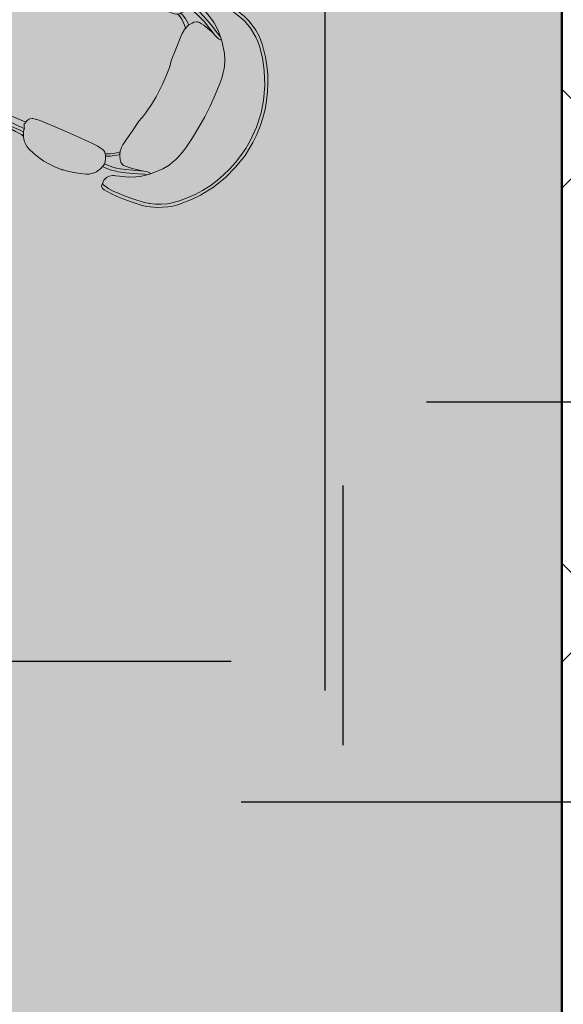
# Model space of a CAD drawing. Units: inches. Extents: x -466983 to 1020, y 324 to 318697.
# Tile 13 of 97: x 794 to 814, y 417 to 452. Entities that reach past the tile are written whole.
import ezdxf

# ---------------------------------------------------------------- set-up
doc = ezdxf.new("R2010")
doc.units = ezdxf.units.IN
doc.header["$MEASUREMENT"] = 0
for name, color, linetype, lineweight in [('A-ANNO-DIMS', 2, 'Continuous', 18), ('A-FLOR-PATT', 252, 'Continuous', 13), ('A-FURN', 8, 'Continuous', 18), ('A-WALL', 7, 'Continuous', 50)]:
    doc.layers.add(name, color=color, linetype=linetype, lineweight=lineweight)
doc.layers.add('K-Hatch', color=7, linetype='Continuous')
doc.styles.get("Standard").update_dxf_attribs({"font": 'arial.ttf'})
doc.dimstyles.get("Standard").update_dxf_attribs({"dimtxt": 6, "dimasz": 4, "dimexe": 3, "dimexo": 3, "dimgap": 0.09, "dimtad": 0, "dimtih": 1, "dimtoh": 1, "dimdec": 1, "dimzin": 0, "dimdsep": 46, "dimlunit": 3, "dimtxsty": 'Standard', "dimcen": 0.09, "dimadec": 0, "dimazin": 0, "dimtfac": 1, "dimtdec": 1, "dimtofl": 0, "dimtmove": 0, "dimatfit": 3, "dimfxl": 1, "dimtolj": 1, "dimtzin": 0, "dimarcsym": 0})

# ---------------------------------------------------------------- blocks, each defined once
blk = doc.blocks.new('CBV_11')
at = {"layer": 'K-Hatch'}
h = blk.add_hatch(color=256, dxfattribs=at)
h.dxf.hatch_style = 1
h.paths.add_polyline_path([(-178.4, 698.3), (-200.4, 717.9), (-207.1, 720), (-213, 721.7), (-231.8, 722.5), (-254.2, 721.5), (-275, 717.7), (-289.3, 712.5), (-316, 699.4), (-324.9, 694.8), (-295.8, 706.5), (-286.8, 709.3), (-277.1, 712.2), (-265.3, 715), (-258.1, 715.9), (-241.3, 718.1), (-228.8, 718), (-215.5, 715.7), (-208.8, 713.2), (-205.5, 711.6), (-203.9, 710.6), (-202.4, 709.7), (-195.4, 705.2), (-194.8, 704.5), (-190.4, 699.8), (-87.3, 570), (16.1, 440.3), (19.6, 435), (22.9, 426.4), (24.1, 422.9), (25.8, 412.3), (25.1, 398.9), (24.2, 394.5), (25.6, 399.8), (28.8, 418.8), (27.5, 432), (13.6, 457)])
h.paths.add_polyline_path([(-536, 213.1), (-639.3, 342.7), (-642.9, 348.1), (-646.2, 356.7), (-647.4, 360.2), (-649.1, 370.8), (-648.4, 384.2), (-645.7, 396.4), (-637.3, 419.1), (-631.8, 430), (-626.9, 438.8), (-622.1, 446.9), (-606.5, 469.3), (-631, 439.9), (-638.6, 427.4), (-646.5, 408.6), (-652.3, 388), (-655.6, 368.8), (-654.4, 355.7), (-649, 343.1), (-640.5, 330.7), (-448.6, 89.4), (-437.6, 77.7), (-424.8, 69.2), (-413.8, 65.9), (-392.4, 64.7), (-388.1, 65), (-394.5, 65), (-407.8, 67.4), (-417, 71.1), (-420.9, 73.4), (-427.9, 77.9), (-428.5, 78.6), (-432.9, 83.2)])
for p, q in [((259, 150.4), (259, 150.4)), ((345.2, 98.6), (344, 99.3)), ((349.3, 96), (349.2, 96.1)), ((478.6, -6.2), (478.7, -6.3)), ((644.9, -391.7), (644.8, -391.9)), ((-99, -470.6), (-98.6, -470.7)), ((4, -570.8), (3.9, -570.4)), ((96.9, -581.8), (98.6, -582.5)), ((157.6, -594.8), (157.4, -595)), ((239.9, -716.7), (240.2, -716.7))]:
    blk.add_line(p, q)
for points in [[(-16.4, 313.8), (-16.1, 314.2), (2.3, 340.9), (8.8, 352.7), (9, 353), (14.8, 365.2), (18.6, 375.8), (20.5, 381.1), (22.4, 386.6), (24.2, 394.5), (25.1, 398.9), (25.8, 412.3), (24.1, 422.9), (22.9, 426.4), (19.6, 435), (16.1, 440.3), (-87.3, 570), (-190.4, 699.8), (-194.8, 704.5), (-195.4, 705.2), (-202.4, 709.7), (-203.9, 710.6), (-208.8, 713.2), (-215.5, 715.7), (-228.8, 718), (-241.3, 718.1), (-258.1, 715.9), (-265.3, 715), (-277.1, 712.2), (-286.8, 709.3), (-295.8, 706.5), (-324.9, 694.8), (-347.4, 685.7), (-397.3, 660.4), (-444.8, 630.8), (-480.8, 604.2), (-497.4, 590.5), (-534.5, 556.2), (-554.4, 535.5), (-590.2, 492.6), (-603.5, 473.5), (-606.5, 469.3), (-622.1, 446.9), (-626.9, 438.8), (-631.8, 430), (-637.3, 419.1), (-645.7, 396.4), (-648.4, 384.2), (-649.1, 370.8), (-647.4, 360.2), (-646.2, 356.7), (-642.9, 348.1), (-639.3, 342.7), (-536, 213.1), (-432.9, 83.2), (-428.5, 78.6), (-427.9, 77.9), (-420.9, 73.4), (-417, 71.1), (-407.8, 67.4), (-394.5, 65), (-388.1, 65), (-382, 64.9), (-376.6, 65.6), (-368.3, 66.6), (-367.7, 66.7), (-359.3, 67.5), (-346.5, 70.4), (-345.9, 70.6), (-336.1, 73.3), (-327.3, 76.2), (-282.4, 94.4), (-275.6, 97.1), (-225.7, 122.4), (-178.3, 151.9), (-142.2, 178.6), (-125.6, 192.2), (-88.5, 226.6), (-68.7, 247.3), (-32.9, 290.2), (-16.4, 313.8), (-16.2, 314.2)], [(9, 353), (10.3, 354.9), (16.2, 365.1), (21.5, 376.3), (26.2, 388.3), (30.1, 400.3), (33.2, 412.3), (35.5, 424.1), (35.7, 431), (33.5, 442.1), (26.2, 456.4), (21.3, 463.1), (-173.2, 707.5), (-185, 718.7), (-200.1, 726), (-205.3, 726.9), (-216.4, 727.2), (-226.1, 726.9), (-241.2, 725.8), (-253.7, 723.9), (-264.9, 721.5), (-277.2, 717.9), (-288.3, 713.3), (-311.8, 701.8), (-324.9, 694.8), (-316, 699.4), (-289.3, 712.5), (-275, 717.7), (-254.2, 721.5), (-231.8, 722.5), (-213, 721.7), (-207.1, 720), (-200.4, 717.9), (-178.4, 698.3), (13.6, 457), (27.5, 432), (28.8, 418.8), (25.6, 399.8), (24.2, 394.5)], [(-203.9, 710.6), (-205.5, 711.6), (-208.8, 713.2)], [(-346.5, 70.4), (-349.3, 69.2), (-356.8, 67), (-372.9, 63.3), (-385.5, 61.5), (-398.1, 60.5), (-410.3, 60.2), (-421.5, 60.6), (-428.5, 61.9), (-441.8, 68.9), (-453.7, 80.2), (-456.3, 83.2), (-648.2, 324.6), (-653.1, 331.3), (-657.2, 338.3), (-662.3, 353.4), (-662.3, 363.4), (-659.9, 375.1), (-656.8, 387), (-652.8, 399), (-648.1, 410.9), (-642.7, 422.1), (-636.8, 432.3), (-630.4, 441.2), (-607, 469.6), (-603.5, 473.5)], [(-606.5, 469.3), (-631, 439.9), (-638.6, 427.4), (-646.5, 408.6), (-652.3, 388), (-655.6, 368.8), (-654.4, 355.7), (-649, 343.1), (-640.5, 330.7), (-448.6, 89.4), (-437.6, 77.7), (-424.8, 69.2), (-413.8, 65.9), (-392.4, 64.7), (-388.1, 65)], [(-50.1, 67.5), (-23.5, 87.9), (-9.9, 97.6), (3.8, 107.1), (17.8, 116.4), (31.9, 125.3), (60.6, 142.4), (89.9, 158.3), (119.5, 173.3), (135, 179.9), (142.8, 182.8), (151, 184.8), (159.6, 185.9), (175.9, 186.9), (181, 186.7)], [(46.8, 133.3), (53.6, 137.3), (58.1, 140), (60.8, 141.6), (71.5, 147.3), (71.5, 147.3), (75.4, 149.5), (86.9, 155.7), (90, 157.4), (100.5, 162.5), (100.5, 162.6), (112.3, 168.5), (118.5, 171.5), (121.5, 172.9), (121.5, 172.9), (121.6, 172.9), (124.8, 174.4), (126.7, 175.2), (131.7, 177.5), (133.5, 178.2), (133.6, 178.2), (139.5, 180.3), (143.1, 181.6), (144.9, 182), (148.5, 182.9), (151.1, 183.5), (151.4, 183.6), (155.5, 184.6), (157.4, 184.8), (163.9, 185.7), (168.2, 186.2), (170.2, 186.3), (175.4, 186.4), (175.6, 186.4), (175.8, 186.4), (179.6, 186.5), (181.7, 186.3), (187.4, 185.9), (192.1, 185.5), (192.4, 185.5), (192.9, 185.4), (196.6, 184.9), (199.1, 184.5), (203, 183.5), (203.6, 183.4), (204.9, 183.1), (206.1, 182.8), (206.2, 182.8), (206.9, 182.5), (210.6, 181.4), (212.8, 180.8), (213.1, 180.7), (213.6, 180.5), (215.8, 179.8), (217.2, 179.4), (219, 178.7), (225, 176.1), (225.2, 176), (225.4, 175.9), (228.9, 174.4), (230.6, 173.5), (239.3, 168.6), (259, 150.4), (261.9, 146.4), (265.2, 141.7), (271.3, 132.8), (271.8, 133.4)], [(268, 169.8), (264.7, 172.2), (256.3, 176.5), (245.7, 180.3), (233.5, 183.5), (219.5, 185.8), (204.9, 187.1), (190.5, 187.3), (181, 186.7), (184.6, 186.6), (192.1, 185.5)], [(215.8, 179.8), (224.2, 178.5), (244.5, 172), (258.1, 164.6), (259.6, 163.4)], [(325.2, 88.8), (320.7, 95.5), (312.8, 106.8), (299.7, 124.6), (287.2, 140.3), (277.4, 151.6), (268.4, 160.4), (262.4, 164.5), (259.6, 163.6), (268, 169.8), (268.8, 170.4), (273.2, 169.7), (281.2, 162.9), (287.4, 156.5), (292.6, 150.4), (299.8, 141.9), (315.6, 121.4), (329.6, 101.6), (335.5, 92.9)], [(259.6, 163.6), (259.6, 163.4), (260.3, 157.9), (264.5, 147.6), (271, 134.8), (273.6, 130.4), (280, 119.4), (306, 80.1)], [(58.1, 140), (55.3, 138.4), (46.8, 133.3), (43.3, 131.2), (32.8, 125), (30.4, 123.5), (28, 122), (23.4, 119.1), (14, 112.9), (5.4, 107.3), (1.3, 104.5), (-2.9, 101.6), (-9.4, 97), (-9.5, 96.9), (-21, 88.8), (-24.8, 86), (-28.5, 83.3), (-36.4, 77.2), (-38.8, 75.4), (-45.1, 70.6), (-49.7, 67), (-54.2, 63.4), (-56, 61.9), (-62.5, 56.6), (-75.5, 45.6), (-77.3, 44), (-77.4, 44)], [(346.5, 95.7), (344, 99.3), (342.7, 101.1), (342.4, 101.6), (329.1, 118.9), (319.4, 130.1), (312.4, 136.8), (292.6, 150.4)], [(457.4, -155.4), (455.9, -155.5), (454.8, -155.5), (454.6, -155.5), (454.5, -155.5), (450.3, -155.2), (448.8, -154.8), (444.9, -153.5), (441.6, -151.7), (437.3, -148.8), (429.3, -140.4), (425.9, -136.3), (421.6, -130.7), (411.3, -116.8), (398.5, -99.2), (386.7, -82.7), (374.5, -65.3), (362.5, -47.8), (339.1, -12.8), (318.2, 19.8), (307.7, 36.3), (302.4, 46.9), (301.4, 48.8), (298.5, 55.5), (297.9, 58.1), (297.8, 65.2), (298.5, 67.6), (301, 75.1), (306, 80.1), (307.5, 81.6), (308.1, 82), (307.8, 84), (308.9, 85.7), (310.4, 86.8), (312.8, 87.1), (320.3, 87.9), (323, 87.9), (324.8, 88.6), (325.2, 88.8), (330.7, 91.3), (335.5, 92.9), (337.7, 93.7), (344.7, 95.5), (346.5, 95.7), (349.3, 96), (349.8, 96), (359.2, 96.9), (368.2, 95.8), (377.2, 93.8), (385.7, 90.7), (393.6, 86.2), (410.4, 73.5), (416, 68.7), (426.3, 59.8), (441.3, 45.2), (454.8, 29), (467.2, 12.1), (478.3, -5.7), (478.6, -6.2), (478.6, -6.3), (479, -7), (481, -10.8), (488.2, -24.1), (496, -43.4), (503.1, -63.4), (508.5, -83.5), (509.8, -91.8), (509.7, -100.3), (508.6, -108.6), (506.6, -116.7), (503.3, -124.2), (500, -131.2), (494.1, -139.1), (490.8, -143.5), (486.4, -147), (485.6, -147.6), (485.6, -147.6)], [(349.8, 96), (347.9, 98), (342.9, 101.1), (342.7, 101.1)], [(-217.7, -216.8), (-218.7, -214.8), (-221.6, -206), (-223.5, -195.1), (-224.4, -170.3), (-223.2, -156.5), (-220.9, -142.4), (-219, -134.5), (-218.9, -134.4), (-218.9, -134.2), (-217.3, -125.9), (-215.2, -117.7), (-212.7, -109.9), (-212.1, -108.4), (-207.7, -98.2), (-203.6, -90.8), (-196.4, -80.6), (-191.3, -74), (-180.9, -61.1), (-170.2, -48.3), (-159.1, -35.9), (-159.1, -35.8), (-148, -23.5), (-124.9, 0.7), (-113, 12.4), (-100.8, 23.9), (-88.5, 35.1), (-75.9, 46.2), (-63.1, 57), (-50.1, 67.5)], [(-214.7, -118), (-214.6, -117.8), (-212.4, -111.4), (-210.9, -107.7), (-210.4, -106.5), (-210.1, -105.7), (-209.4, -104.2), (-209, -103.5), (-206, -97.3), (-205.1, -95.8), (-204.7, -95), (-203.9, -93.8), (-203.5, -93.2), (-202.6, -91.5), (-202, -90.5), (-200.3, -88.1), (-199.3, -86.6), (-198.2, -84.9), (-198, -84.7), (-197.9, -84.5), (-192.8, -77.9), (-190.9, -75.4), (-190.5, -74.9), (-189.8, -74), (-186.5, -69.8), (-173.8, -54.2), (-170.7, -50.6), (-169.2, -48.8), (-167, -46.3), (-160.8, -39.1), (-147.5, -24.2), (-147.4, -24.1), (-147.3, -24), (-146.9, -23.6), (-146.4, -23.1), (-134, -9.8), (-127, -2.7), (-124.7, -0.3), (-124.4, -0.1), (-124.2, 0.2), (-123.2, 1.2), (-120.2, 4.2), (-106.2, 17.9), (-102.9, 20.9), (-101.4, 22.4), (-98.9, 24.6), (-91.9, 31.1), (-77.7, 43.7), (-77.6, 43.8), (-77.4, 44)], [(479, -7), (479.3, -7.2), (478.7, -6.3), (478.6, -6.3)], [(481, -10.8), (480.9, -9.4), (480, -8.1), (479.3, -7.2), (479.9, -7.7), (480, -8.1), (480, -8.6)], [(-212.1, -108.4), (-213.8, -111.2), (-223, -134.4), (-228.6, -157.2), (-231.3, -180.4), (-231, -201.3), (-228.1, -217.6), (-225.8, -223.3), (-226.1, -223.6), (-227.6, -226.1), (-224.9, -232.9), (-218.3, -243.6), (-212.6, -251.5), (-209.6, -255.8), (-197.1, -271.4), (-182.6, -288.2), (-173.4, -298.4), (-166.3, -306.1)], [(-143.8, -278.1), (-149.7, -271.9), (-151.2, -270.2), (-153.6, -267.6), (-153.7, -267.6), (-158.2, -262.7), (-179.1, -240.4), (-181.9, -237.4), (-184, -235.2), (-185.8, -233.2), (-188.4, -230.4), (-188.8, -230), (-189.2, -229.5), (-191, -227.5), (-192.6, -225.7), (-192.9, -225.2), (-193.3, -224.8), (-194.6, -223.3), (-196.5, -221), (-197, -220.3), (-197.5, -219.7), (-198.5, -218.3), (-200, -216.4), (-200.2, -216.2), (-201.3, -214.6), (-201.4, -214.5), (-203.2, -212), (-203.8, -211.2), (-204.4, -210.2), (-205.3, -208.8), (-206.1, -207.6), (-206.2, -207.4), (-206.3, -207.3), (-206.4, -207), (-206.6, -206.8), (-207.1, -206), (-207.5, -205.3), (-207.5, -205.2), (-207.6, -205.1), (-207.6, -205), (-208.1, -204.2), (-208.2, -204), (-208.3, -203.8), (-208.4, -203.7), (-208.7, -203.2), (-209.4, -202), (-209.4, -201.9), (-209.6, -201.7), (-210.3, -200.2), (-211.3, -198.2), (-211.5, -197.7), (-212.6, -194.8), (-213.7, -191.8), (-214, -190.9), (-215.6, -185.2), (-217, -180.3), (-217, -180.3), (-217, -180.3), (-217.6, -177.7), (-218.5, -172.7), (-218.9, -170.6), (-219, -169.1), (-219.2, -168.2), (-219.2, -167.9), (-219.3, -167.8), (-219.3, -166.9), (-219.6, -165), (-219.8, -163.4), (-220.2, -156.1), (-220.2, -148.7), (-219.6, -142.8), (-219.6, -142.2), (-219.6, -142), (-219.6, -141.7), (-219.5, -141.2), (-218.5, -134), (-217.9, -130.8), (-217.7, -129.5), (-217.7, -129.3), (-217.5, -128.7), (-217.5, -128.6), (-217.4, -128.4), (-217, -126.3), (-215, -118.8), (-214.9, -118.6), (-214.9, -118.5), (-214.7, -118), (-214.9, -118.5)], [(2.4, -563.5), (-3.3, -568.8), (-5, -573.7), (-2.4, -580.9), (5.2, -592.9), (5.7, -593.8), (18.8, -610.1), (45.9, -638.4), (68.4, -659.3), (96.5, -683.5), (112.7, -694.7), (124, -701.1), (147.3, -712), (166.9, -718.5), (179.8, -721.6), (199.9, -724.8), (239.8, -727.2), (268.3, -726.6), (296.4, -724), (325.3, -719.4), (352.9, -713), (380.3, -704.7), (407.4, -694.3), (433.1, -682.4), (458.3, -668.7), (482.6, -653.1), (505.7, -636), (542.7, -602.8), (575.4, -565.6), (602.5, -526.6), (625.7, -483.1), (643.9, -436.4), (652.7, -404.6), (661, -358.1), (662.3, -341.6), (662.3, -324.4), (657.8, -289.7), (648.3, -258), (641.9, -243.3), (624.1, -210.4), (611.5, -188.5), (598.9, -168.7), (586.8, -151.4), (569.2, -131.1), (563.8, -126.7), (556, -124), (545.5, -130.4)], [(155.2, -596.2), (151.6, -595.8), (147.4, -595.1), (129.4, -592.1), (123.7, -590.8), (98.6, -582.5), (97.8, -582.2), (96.9, -581.8), (74.8, -570.5), (62.9, -563.8), (52.4, -557.5), (46.9, -554.5), (42.7, -553), (37.7, -551.6), (36.8, -551.4), (31.7, -550), (21.6, -550.8), (19.3, -551.6), (10.7, -555.3), (9.9, -555.9), (4.7, -561.9), (2.4, -563.5), (3.7, -570.3), (4, -570.8), (6.8, -576.4), (8.9, -579.3), (10.2, -583.1), (17.3, -590.8), (22.7, -598.1), (36.7, -613.8), (53.2, -630.5), (71.6, -647.7), (77.1, -652.5), (77.9, -653.2), (88.3, -662.3), (97.4, -670.5), (112.3, -681.7), (138.1, -696.5), (170, -708.5), (185.7, -712.2), (201.4, -714.5), (240.2, -716.9), (281.9, -715.3), (330.8, -707.8), (377.8, -694.8), (416.2, -679.4), (459.2, -656.3), (499.4, -628.1), (521, -609.6), (541.3, -589.7), (560.1, -568.5), (577.1, -546.4), (593, -522.5), (607, -498.1), (619.2, -472.7), (629.8, -445.9), (638.3, -419.5), (645, -392), (649.6, -365.8), (651.8, -341.4), (651.9, -325.2), (649.9, -305.2), (646.3, -287), (640.9, -268.7), (640.2, -267.3), (639, -264.2), (633.6, -250.9), (617.4, -220.5), (602.1, -193.8), (587.3, -171.3), (580.6, -161.1), (567.7, -144.8), (566, -143.1), (564.1, -141.2), (554.6, -132.1), (554, -131.9), (550.5, -130.5), (549.7, -130.2), (547.6, -129.3), (545.5, -130.4), (545.4, -130.9), (538.4, -135.5), (532.9, -143.1), (531.5, -145.1), (528.5, -154.8), (529, -166.6), (529.5, -170.7), (531.1, -176.4), (534.9, -188.3), (538.2, -199.2), (543, -215.6), (547.1, -240.2), (547.6, -254.2), (546.4, -277.3), (546.2, -281.9), (545.7, -285.4), (545.4, -287.9), (545.4, -287.9), (545.3, -288.8), (545.3, -289.2), (544.3, -296.8), (542.7, -303.6), (537, -331.4), (528.9, -353.7)], [(454.6, -155.5), (454.7, -155.7), (455.1, -157.8), (455.5, -160), (455.6, -160.6), (455.6, -160.7), (456.7, -166.6), (457.5, -171.5), (458.2, -182.7), (458.6, -192.3), (458.1, -202.7), (457.9, -204.1)], [(457.4, -155.4), (457.4, -155.4), (466.4, -154.5), (471.9, -153.3), (475.6, -151.4), (481.8, -150.7), (486.4, -147), (489.4, -151.4), (501.8, -172.4), (506.9, -183.2), (511.5, -194.8), (517.3, -212.7), (523.5, -234.6), (529.9, -258.9), (536.2, -278.2), (545.2, -290)], [(461.9, -154.9), (462.2, -156.4), (462.6, -158.7), (462.7, -159.1), (462.7, -159.3), (463.8, -165.3), (464.7, -170.7), (465.4, -182.4), (465.8, -192.3), (465.4, -201.6)], [(494.1, -139.1), (498.2, -145.2), (508.4, -161.7), (516.9, -179.1), (519.8, -186.7), (527.6, -210), (534, -233), (538.1, -249.1), (543.9, -270.8), (546.4, -277.4)], [(549.7, -130.2), (547, -129.8), (545.4, -130.9)], [(-225.8, -223.3), (-218.8, -216.5), (-217.7, -216.8), (-213.1, -218.1), (-195.7, -231.2), (-175.3, -250.4), (-147.2, -280.1)], [(-159.9, -297.1), (-165.4, -291.2), (-181.5, -273.1), (-197.1, -254.2), (-203.8, -245.5), (-213.9, -230.9), (-219, -220.9), (-218.8, -216.5)], [(-212.6, -251.5), (-211.9, -253), (-204.6, -272.1), (-201.7, -277.7), (-192.5, -291.1), (-180.6, -305.8), (-175.6, -311.7), (-173.4, -314.3), (-171.3, -316.5)], [(49.6, -472.3), (49.5, -472.3), (49.1, -466.8), (46.3, -459.7), (42.7, -453.8), (36.7, -445.8), (32.2, -440.3), (21, -427.2), (-6.6, -395.6), (-20.8, -379.7), (-35.2, -364.1), (-64.1, -333.5), (-77.2, -319.8), (-92.5, -304.3), (-108.7, -288.6), (-115.6, -282.9), (-121.5, -278.5), (-131.9, -275.3), (-141.2, -276.5), (-143.8, -278.1), (-147.2, -280.1), (-148.4, -280.8), (-149.5, -281.9), (-150.1, -282.4), (-156.3, -292.9), (-159.1, -296.2), (-158.4, -292.9), (-155.5, -285.3), (-153.9, -281.9), (-151.3, -281.2), (-149.5, -281.9)], [(545.7, -285.4), (544.3, -287.1), (544, -287.5), (543.6, -287.7), (543.5, -287.7)], [(59.4, -477), (56.9, -476.1), (53.2, -474.4), (49.6, -472.8), (49.7, -473.8), (48.7, -479.4), (48, -481.2), (44.9, -489.9), (42.9, -494.4), (41, -497.8), (38.6, -502.4), (37.3, -504.2), (36.9, -504.7), (34.8, -506.8), (33.8, -507.4), (29.1, -510.5), (24.1, -512.8), (22.1, -513.7), (15.1, -516.8), (-0.5, -520.1), (-9, -519.9), (-17.2, -519.3), (-25.5, -517.5), (-33.3, -514.4), (-51.7, -504.6), (-69.5, -493.5), (-86.6, -481.2), (-95.4, -473.4), (-97.6, -471.5), (-98, -471.2), (-98.6, -470.7), (-101.4, -468.2), (-101.5, -468.1), (-102.3, -467.4), (-117.4, -452.7), (-131.1, -436.8), (-143.6, -419.9), (-154.4, -402.1), (-164.5, -383.6), (-172.5, -364.3), (-175.2, -355.6), (-176.8, -346.5), (-176.8, -337.4), (-175.1, -328.4), (-173.5, -321.4), (-172.7, -319.6), (-171.3, -316.5), (-167.5, -308.1), (-166.3, -306.1), (-163.8, -301.8), (-160.2, -297.5), (-159.9, -297.1), (-159.1, -296.2)], [(-175.6, -311.7), (-175.4, -312.6), (-174, -317.8), (-172.7, -319.6)], [(528.6, -354.6), (528.9, -353.7), (522.8, -365.4), (515.7, -377.3), (508.1, -388.2), (503.2, -394.5), (496, -403.1), (483, -417.1), (469.3, -430.9), (454.9, -444.7), (425.1, -471.8), (395, -496.8), (363.8, -520.6), (330.7, -543.5), (314.1, -554.4), (297.5, -564.7), (281, -574.1), (263.9, -582.5), (251.4, -587.6), (244.7, -589.7), (224.5, -595.3), (204.1, -597.7), (165.9, -597.3), (155.2, -596.2), (157.4, -595), (157.2, -592.9), (152.6, -587.1)], [(-101.4, -468.2), (-100.6, -469.4), (-101.3, -468.7), (-101.5, -468.1)], [(-98, -471.2), (-98.4, -471.1), (-98.9, -470.8), (-99.9, -470.3), (-100.5, -469.5), (-100.6, -469.4)], [(-97.6, -471.5), (-98.3, -471.4), (-98.9, -470.8)], [(90.8, -500.6), (86.1, -499.5), (84, -498.9), (73.3, -495), (70.3, -493.8), (55.2, -486.1), (48, -481.2)], [(99.2, -488.5), (98.9, -488.4), (88.6, -486.6), (78.5, -484.1), (68.6, -480.9), (59.4, -477), (58.2, -476.5), (57.8, -476.3), (49.6, -472.3), (49.6, -472.3), (49.6, -472.4), (49.6, -472.4), (49.6, -472.5), (49.6, -472.8)], [(147.4, -595.1), (145, -593.4), (134.3, -587.3), (109, -574.1), (88.3, -563.1), (68.7, -551.4), (57.7, -543.9), (47.9, -536.1), (44.1, -532.6), (29.2, -518.3), (24.1, -512.8), (24.1, -512.8)], [(33.8, -507.4), (37.2, -511.1), (50.6, -524.3), (64.4, -535.5), (70.8, -539.8), (90.6, -552.1), (111.2, -563.3), (124.8, -570.5), (137.6, -577.4), (152.6, -587)]]:
    blk.add_lwpolyline(points)
blk.add_lwpolyline([(536.2, -278.2, 0.060196), (503, -207.6), (501.6, -205.9), (497.9, -203.4), (490.4, -200.5), (481.7, -199.9), (471.1, -200.5), (466.7, -201.3), (465.7, -201.5), (464.5, -201.7), (461.1, -203), (457.9, -204.1), (457.5, -204.3), (457.5, -204.3), (454.5, -205.4), (446.6, -210), (444.1, -211.8), (435.9, -217.8), (427.5, -225.4), (419.3, -234.2), (396.7, -256.7), (369.9, -282.9), (360.7, -294.8), (359, -297.1), (344.2, -313.2), (323.9, -333.2), (301.6, -353), (288.9, -363.5), (265.5, -381.1), (241.1, -397.6), (216.3, -412.6), (192.3, -424.2), (160.7, -444.5), (123.2, -467.5), (113.9, -474), (106.2, -480.6), (103.9, -482.6), (100.1, -487.3), (99.2, -488.5), (96.5, -492), (94.1, -495.1), (91.8, -498.2), (91.4, -499.3), (90.8, -500.6), (90.3, -501.9), (88.1, -510.2), (87, -512.3), (85.3, -518.2), (85.1, -527), (85.8, -529.8), (88.9, -536.1, 0.065332), (140.4, -579.1)], format="xyb")
blk = doc.blocks.new('Garden Sofa')
at = {"xscale": -0.0109740885734132, "yscale": 0.0109740885734132, "zscale": 0.0109740885734132, "rotation": 100.5267845499335}
blk.add_blockref('CBV_11', (2467.574, 814.959), dxfattribs=at)
blk = doc.blocks.new('*D93')
at = {"layer": 'A-ANNO-DIMS', "color": 0, "lineweight": -2, "transparency": 16777216}
for p, q in [((808.966, 500.777), (818.266, 500.777)), ((815.266, 496.777), (815.266, 472.969)), ((815.266, 442.777), (815.266, 466.584)), ((808.966, 438.777), (818.266, 438.777))]:
    blk.add_line(p, q, dxfattribs=at)
at = {"layer": 'A-ANNO-DIMS', "color": 0, "transparency": 16777216}
for points in [[(814.599, 496.777), (815.933, 496.777), (815.266, 500.777)], [(814.599, 442.777), (815.933, 442.777), (815.266, 438.777)]]:
    blk.add_solid(points, dxfattribs=at)
at = {"layer": 'Defpoints', "color": 0, "transparency": 16777216}
for p in [(805.966, 500.777), (815.266, 500.777), (805.966, 438.777)]:
    blk.add_point(p, dxfattribs=at)
at = {"layer": 'A-ANNO-DIMS', "color": 0, "transparency": 16777216, "insert": (815.266, 469.777), "char_height": 6, "attachment_point": 5}
blk.add_mtext('\\A1;GARDEN SEAT 62', dxfattribs=at)
blk = doc.blocks.new('*D94')
at = {"layer": 'A-ANNO-DIMS', "color": 0, "lineweight": -2, "transparency": 16777216}
for p, q in [((753.135, 435.777), (753.135, 426.477)), ((805.966, 435.777), (805.966, 426.477)), ((757.135, 429.477), (775.163, 429.477)), ((801.966, 429.477), (783.938, 429.477))]:
    blk.add_line(p, q, dxfattribs=at)
at = {"layer": 'A-ANNO-DIMS', "color": 0, "transparency": 16777216}
for points in [[(757.135, 430.143), (757.135, 428.81), (753.135, 429.477)], [(801.966, 430.143), (801.966, 428.81), (805.966, 429.477)]]:
    blk.add_solid(points, dxfattribs=at)
at = {"layer": 'Defpoints', "color": 0, "transparency": 16777216}
for p in [(753.135, 438.777), (805.966, 438.777), (805.966, 429.477)]:
    blk.add_point(p, dxfattribs=at)
at = {"layer": 'A-ANNO-DIMS', "color": 0, "transparency": 16777216, "insert": (779.551, 429.477), "char_height": 6, "attachment_point": 5}
blk.add_mtext('\\A1;53', dxfattribs=at)
blk = doc.blocks.new('*D97')
at = {"layer": 'A-ANNO-DIMS', "color": 0, "lineweight": -2, "transparency": 16777216}
for p, q in [((823.929, 568.441), (802.329, 568.441)), ((805.329, 564.441), (805.329, 499.545)), ((805.329, 428.441), (805.329, 493.337)), ((823.929, 424.441), (802.329, 424.441))]:
    blk.add_line(p, q, dxfattribs=at)
at = {"layer": 'A-ANNO-DIMS', "color": 0, "transparency": 16777216}
for points in [[(804.662, 564.441), (805.996, 564.441), (805.329, 568.441)], [(804.662, 428.441), (805.996, 428.441), (805.329, 424.441)]]:
    blk.add_solid(points, dxfattribs=at)
at = {"layer": 'Defpoints', "color": 0, "transparency": 16777216}
for p in [(826.929, 568.441), (805.329, 424.441), (826.929, 424.441)]:
    blk.add_point(p, dxfattribs=at)
at = {"layer": 'A-ANNO-DIMS', "color": 0, "transparency": 16777216, "insert": (805.329, 496.441), "char_height": 6, "attachment_point": 5}
blk.add_mtext('\\A1;BIKE 144', dxfattribs=at)

msp = doc.modelspace()

# ---------------------------------------------------------------- hatches: boundary and pattern name
at = {"layer": 'A-FLOR-PATT', "transparency": 33554572}
h = msp.add_hatch(dxfattribs=at)
h.set_pattern_fill('AR-HBONE', color=256, scale=3)
h.set_pattern_definition([(45, (-1212.414, -290.035), (0, 16.97056), [36, -12]), (135, (-1203.928, -281.55), (1e-15, 16.97056), [36, -12])])
h.paths.add_polyline_path([(987.806, 618.938), (813.806, 618.938), (813.806, 368.938), (987.806, 368.938)])
at = {"layer": 'A-FLOR-PATT', "transparency": 33554661}
h = msp.add_hatch(color=256, dxfattribs=at)
h.dxf.hatch_style = 1
h.set_gradient(color1=(19, 155, 72), color2=(0, 107, 0), name='CYLINDER')
h.paths.add_polyline_path([(813.806, 503.938), (730.806, 503.938), (730.806, 424.938), (612.806, 424.938), (612.806, 415.938), (442.806, 415.938), (442.806, 368.938), (813.806, 368.938)])
h.paths.add_polyline_path([(771.796, 407.07), (783.796, 407.07), (783.796, 371.07), (771.796, 371.07)], flags=16)
h.paths.add_polyline_path([(755.796, 407.07), (755.796, 371.07), (743.796, 371.07), (743.796, 407.07)], flags=16)
h.paths.add_polyline_path([(769.796, 404.07), (769.796, 374.07), (757.796, 374.07), (757.796, 404.07)], flags=16)
h.paths.add_polyline_path([(785.796, 404.07), (797.796, 404.07), (797.796, 374.07), (785.796, 374.07)], flags=16)
h.paths.add_polyline_path([(741.796, 404.07), (741.796, 374.07), (729.796, 374.07), (729.796, 404.07)], flags=16)
h.paths.add_polyline_path([(799.796, 407.07), (811.796, 407.07), (811.796, 371.07), (799.796, 371.07)], flags=16)
h.paths.add_polyline_path([(727.796, 407.07), (727.796, 371.07), (715.796, 371.07), (715.796, 407.07)], flags=16)
h.paths.add_polyline_path([(713.796, 404.07), (713.796, 374.07), (701.796, 374.07), (701.796, 404.07)], flags=16)
h.paths.add_polyline_path([(699.796, 407.07), (699.796, 371.07), (687.796, 371.07), (687.796, 407.07)], flags=16)
h.paths.add_polyline_path([(685.796, 404.07), (685.796, 374.07), (673.796, 374.07), (673.796, 404.07)], flags=16)
h.paths.add_polyline_path([(671.796, 407.07), (671.796, 371.07), (659.796, 371.07), (659.796, 407.07)], flags=16)
h.paths.add_polyline_path([(657.796, 404.07), (657.796, 374.07), (645.796, 374.07), (645.796, 404.07)], flags=16)
h.paths.add_polyline_path([(643.796, 407.07), (643.796, 371.07), (631.796, 371.07), (631.796, 407.07)], flags=16)
h.paths.add_polyline_path([(629.796, 404.07), (629.796, 374.07), (617.796, 374.07), (617.796, 404.07)], flags=16)
h.paths.add_polyline_path([(615.796, 407.07), (615.796, 371.07), (603.796, 371.07), (603.796, 407.07)], flags=16)
h.paths.add_polyline_path([(601.796, 404.07), (601.796, 374.07), (589.796, 374.07), (589.796, 404.07)], flags=16)
at = {"layer": 'A-FLOR-PATT'}
h = msp.add_hatch(dxfattribs=at)
h.set_pattern_fill('GRASS', color=256, scale=6)
h.set_pattern_definition([(90, (-1212.4137, -290.035), (-4.242641, 4.242641), [1.125, -7.360281]), (45, (-1212.4137, -290.035), (-4.24264, 4.24264), [1.125, -4.875]), (135, (-1212.4137, -290.035), (-4.24264, -4.24264), [1.125, -4.875])])
h.paths.add_polyline_path([(813.806, 503.938), (730.806, 503.938), (730.806, 424.938), (612.806, 424.938), (612.806, 415.938), (442.806, 415.938), (442.806, 368.938), (813.806, 368.938)])
h.paths.add_polyline_path([(589.796, 404.07), (601.796, 404.07), (601.796, 374.07), (589.796, 374.07)], flags=16)
h.paths.add_polyline_path([(603.796, 407.07), (615.796, 407.07), (615.796, 371.07), (603.796, 371.07)], flags=16)
h.paths.add_polyline_path([(617.796, 404.07), (629.796, 404.07), (629.796, 374.07), (617.796, 374.07)], flags=16)
h.paths.add_polyline_path([(631.796, 407.07), (643.796, 407.07), (643.796, 371.07), (631.796, 371.07)], flags=16)
h.paths.add_polyline_path([(645.796, 404.07), (657.796, 404.07), (657.796, 374.07), (645.796, 374.07)], flags=16)
h.paths.add_polyline_path([(659.796, 407.07), (671.796, 407.07), (671.796, 371.07), (659.796, 371.07)], flags=16)
h.paths.add_polyline_path([(673.796, 404.07), (685.796, 404.07), (685.796, 374.07), (673.796, 374.07)], flags=16)
h.paths.add_polyline_path([(687.796, 407.07), (699.796, 407.07), (699.796, 371.07), (687.796, 371.07)], flags=16)
h.paths.add_polyline_path([(701.796, 404.07), (713.796, 404.07), (713.796, 374.07), (701.796, 374.07)], flags=16)
h.paths.add_polyline_path([(715.796, 407.07), (727.796, 407.07), (727.796, 371.07), (715.796, 371.07)], flags=16)
h.paths.add_polyline_path([(729.796, 404.07), (741.796, 404.07), (741.796, 374.07), (729.796, 374.07)], flags=16)
h.paths.add_polyline_path([(743.796, 407.07), (755.796, 407.07), (755.796, 371.07), (743.796, 371.07)], flags=16)
h.paths.add_polyline_path([(757.796, 404.07), (769.796, 404.07), (769.796, 374.07), (757.796, 374.07)], flags=16)
h.paths.add_polyline_path([(771.796, 407.07), (783.796, 407.07), (783.796, 371.07), (771.796, 371.07)], flags=16)
h.paths.add_polyline_path([(785.796, 404.07), (797.796, 404.07), (797.796, 374.07), (785.796, 374.07)], flags=16)
h.paths.add_polyline_path([(799.796, 407.07), (811.796, 407.07), (811.796, 371.07), (799.796, 371.07)], flags=16)

# ---------------------------------------------------------------- linework, layer by layer
at = {"layer": 'A-WALL'}
msp.add_line((813.806, 618.938), (813.806, 368.938), dxfattribs=at)

# ---------------------------------------------------------------- block references
at = {"layer": 'A-FURN'}
msp.add_blockref('Garden Sofa', (-1672.7, -362.711), dxfattribs=at)

# ---------------------------------------------------------------- dimensions: what is measured, and where the dimension line sits
at = {"layer": 'A-ANNO-DIMS'}
for base, p1, p2, angle, text, picture, middle in [((805.329, 424.441), (826.929, 568.441), (826.929, 424.441), 270, 'BIKE <>', '*D97', (805.329, 496.441)), ((815.266, 500.777), (805.966, 438.777), (805.966, 500.777), 90, 'GARDEN SEAT <>', '*D93', (815.266, 469.777))]:
    dim = msp.add_linear_dim(base=base, p1=p1, p2=p2, angle=angle, text=text, dimstyle='Standard', override={"dimdec": 0, "dimlfac": 1, "dimrnd": 0, "dimzin": 0, "dimdsep": 46, "dimlunit": 2}, dxfattribs=at)
    dim.commit()
    dim.dimension.update_dxf_attribs({"geometry": picture, "text_midpoint": middle})
dim = msp.add_linear_dim(base=(805.966, 429.477), p1=(753.135, 438.777), p2=(805.966, 438.777), dimstyle='Standard', override={"dimdec": 0, "dimlfac": 1, "dimrnd": 0, "dimzin": 0, "dimdsep": 46, "dimlunit": 2}, dxfattribs=at)
dim.commit()
dim.dimension.update_dxf_attribs({"geometry": '*D94', "text_midpoint": (779.551, 429.477)})

doc.saveas('drawing.dxf')
